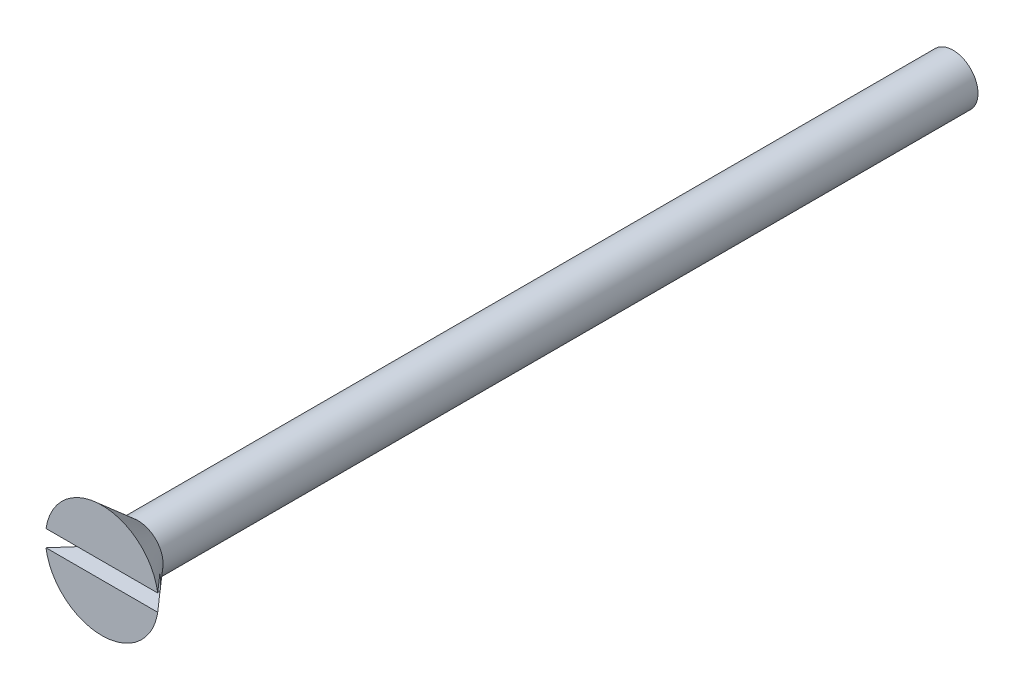
from build123d import *

# Parameters (mm, degrees)
SHANK_PROFILE_0_138_R       = 1.7526
SHANK_0_138_X_2_25_DEPTH    = 57.15
SCREWDRIVER_SLOT_DEPTH      = 60.952219472
SCREWDRIVER_SLOT_DEPTH_BACK = 60.952219472
SCREWDRIVER_SLOT_PROFILE_W  = 2.54
SCREWDRIVER_SLOT_PROFILE_H  = 1.168589104


with BuildPart() as part:
    # Shank Profile Ø0.138 → Shank Ø0.138 x 2.25 (new body)
    with BuildSketch(Plane.XY):
        Circle(SHANK_PROFILE_0_138_R)
    extrude(amount=SHANK_0_138_X_2_25_DEPTH)

    # Countersunk Head Profile → Countersunk Head 82° (revolve)
    with BuildSketch(Plane(origin=(0, 0, 0), x_dir=(0, 0, -1), z_dir=(1, 0, 0)), mode=Mode.PRIVATE) as countersunk_head_82_sk:
        Polygon((-57.15, 1.7526), (-59.69, 3.960588314), (-59.69, 0), (-57.15, 0), align=None)
    revolve(countersunk_head_82_sk.sketch.rotate(Axis((0, 0, 59.69), (0, 0, -1)), 180), axis=Axis((0, 0, 59.69), (0, 0, -1)))

    # Screwdriver Slot Profile → Screwdriver Slot (cut, two sides: drawn at the far end of the back side and taken through both)
    with BuildSketch(Plane(origin=(0, 0, 0), x_dir=(0, 0, -1), z_dir=(1, 0, 0)).offset(-SCREWDRIVER_SLOT_DEPTH_BACK)):
        with Locations((-59.69, 0)):
            Rectangle(SCREWDRIVER_SLOT_PROFILE_W, SCREWDRIVER_SLOT_PROFILE_H)
    extrude(amount=SCREWDRIVER_SLOT_DEPTH + SCREWDRIVER_SLOT_DEPTH_BACK, mode=Mode.SUBTRACT)


solid = part.part
